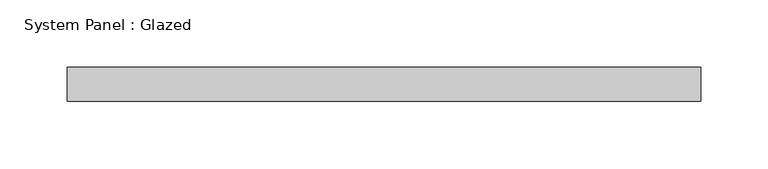
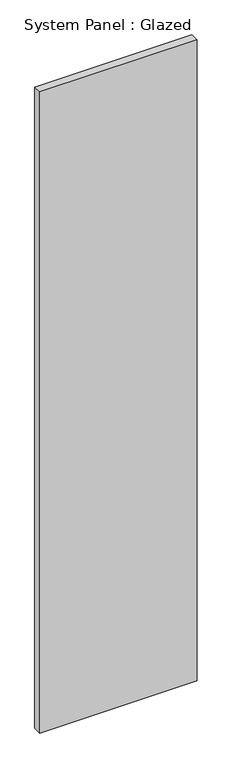
"""IFC4 building model written with IfcOpenShell, lengths in millimetres: plate geometry, System Panel : Glazed."""

from ifc_helpers import new_model, si_unit, origin, origin_with_axes, place, context, project, spatial, polyline, outline, extrude, source, transform, mapped, element, save


def system_panel_glazed_c7815b78(model_context):
    return source(origin(), model_context, "Body", "SweptSolid", [
        extrude(outline(polyline([(235.7662867, 19.05), (-235.7662867, 19.05), (-235.7662867, 44.45), (235.7662867, 44.45), (235.7662867, 19.05)])), origin_with_axes(), (0.0, 0.0, 1.0), 2032.0),
    ])


if __name__ == "__main__":
    model = new_model("IFC4")
    model_context = context("Model", 3, world=origin())
    ifc_project = project(units=[si_unit("LENGTHUNIT", "METRE", prefix="MILLI")], contexts=[model_context])
    site = spatial("IfcSite", under=ifc_project)
    building = spatial("IfcBuilding", under=site)
    placement = place(None, origin())
    system_panel_glazed_shape = system_panel_glazed_c7815b78(model_context)
    element("IfcPlate", 1, ObjectType="System Panel : Glazed", at=placement, inside=building, context=model_context, shape_type="MappedRepresentation", body=[
        mapped(system_panel_glazed_shape, transform((0.0, 0.0, 0.0), x_axis=(1.0, 0.0, 0.0), y_axis=(0.0, 1.0, 0.0), z_axis=(0.0, 0.0, 1.0))),
    ])
    save(model, "model.ifc")

# Revit data of these elements
# Type "System Panel : Glazed"
#   Construction Type Id = "GSP4R"
#   Analytic Construction = "1/8 in Pilkington single glazing"
#   Visual Light Transmittance = 0.9
#   Solar Heat Gain Coefficient = 0.86
#   Heat Transfer Coefficient (U) = 1.18115 BTU/(h·ft²·°F)
# Element 1 (IfcPlate, "System Panel : Glazed")
#   Materials on its faces: "Glass"
# Materials
#   "Glass": class "Glass", colour RGB 0 128 192, transparency 0.75, Description = "Soda Lime Glass", Cost = 0
